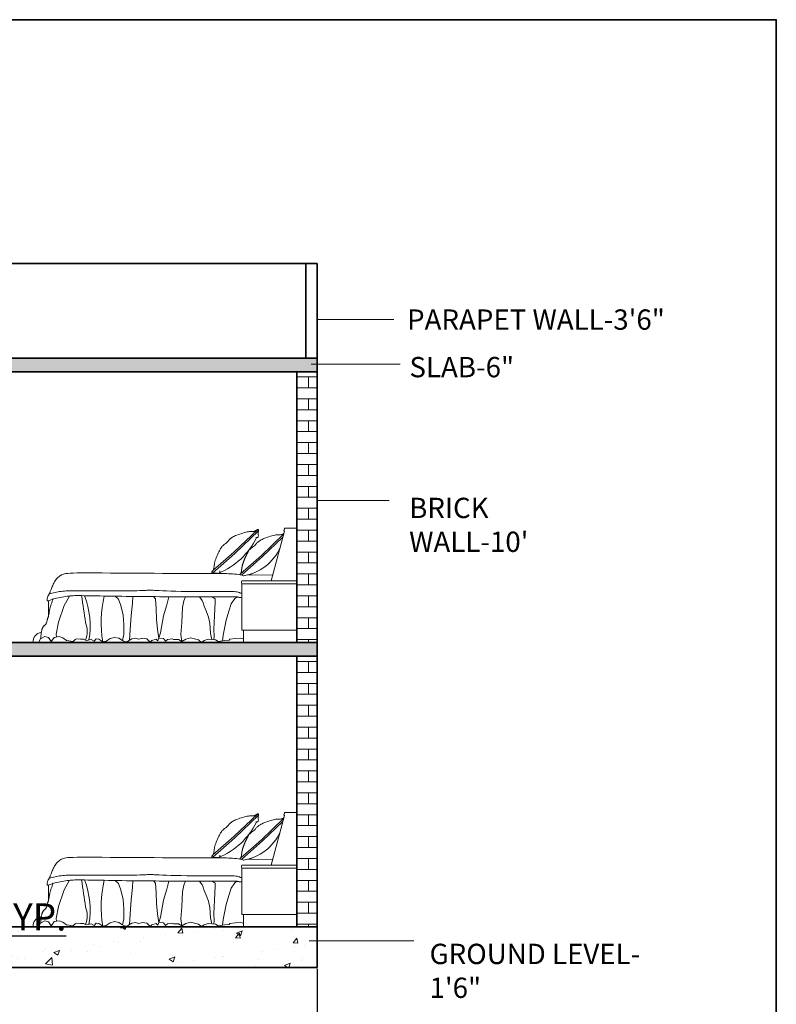
# Model space of a CAD drawing. Units: inches. Extents: x 2142 to 3604, y 1690 to 2981.
# Tile 9 of 9: x 3269 to 3604, y 2545 to 2981. Entities that reach past the tile are written whole.
import ezdxf

# ---------------------------------------------------------------- set-up
doc = ezdxf.new("R2010")
doc.units = ezdxf.units.IN
for name, color, linetype, lineweight in [('A-ANNO-DIMS', 2, 'Continuous', 18), ('A-ANNO-TEXT', 7, 'Continuous', 18), ('A-ANNO-TTLB', 7, 'Continuous', 35), ('A-FLOR-PATT', 8, 'Continuous', 13), ('A-FURN', 8, 'Continuous', 18), ('A-SECT', 7, 'Continuous', 35), ('A-WALL-PATT', 8, 'Continuous', 13)]:
    doc.layers.add(name, color=color, linetype=linetype, lineweight=lineweight)
doc.styles.get("Standard").update_dxf_attribs({"font": 'arial.ttf'})
doc.dimstyles.new('ISO-25', dxfattribs={"dimtxt": 12, "dimasz": 2.5, "dimexe": 1.25, "dimexo": 0.625, "dimtad": 1, "dimdec": 0, "dimlunit": 3, "dimtxsty": 'Standard', "dimcen": 2.5, "dimadec": 0, "dimazin": 0, "dimtfac": 1, "dimtdec": 0, "dimtmove": 0, "dimatfit": 3, "dimfxl": 1, "dimarcsym": 0})

# ---------------------------------------------------------------- blocks, each defined once
blk = doc.blocks.new('A$C08BC4B9A')
for p, q in [((0, 924.5), (0.5, 925)), ((0, 0), (0, 924.5)), ((95, 925), (0.5, 925)), ((101.1, 921.9), (105, 907.4)), ((101.4, 901.2), (208.9, 500)), ((106.6, 881.7), (106.8, 881.6)), ((106.8, 881.6), (109.7, 879.8)), ((109.7, 879.8), (112.8, 878.1)), ((112.8, 878.1), (116.3, 876.5)), ((311.4, 909.3), (311.5, 910.8)), ((311.5, 907.6), (311.4, 909.3)), ((311.5, 910.8), (311.7, 912.1)), ((311.7, 905.6), (311.5, 907.6)), ((311.7, 912.1), (312.1, 913.2)), ((312, 903.5), (311.7, 905.6)), ((502.9, 721.7), (311.9, 904.5)), ((312.3, 901.1), (312, 903.5)), ((312.1, 913.2), (312.7, 914.1)), ((312.6, 898.6), (312.3, 901.1)), ((312.9, 895.9), (312.6, 898.6)), ((312.7, 914.1), (313.6, 914.7)), ((313.1, 892.9), (312.9, 895.9)), ((313.3, 889.8), (313.1, 892.9)), ((313.4, 886.5), (313.3, 889.8)), ((313.3, 875.5), (313.4, 879.4)), ((313.4, 883), (313.4, 886.5)), ((313.4, 879.4), (313.4, 883)), ((313.6, 914.7), (314.7, 915)), ((314.7, 915), (316, 915.1)), ((316, 915.1), (317.6, 914.9)), ((317.6, 914.9), (319.3, 914.5)), ((319.3, 914.5), (321.1, 913.7)), ((511.6, 731.1), (320.5, 913.9)), ((321.1, 913.7), (323.2, 912.6)), ((323.2, 912.6), (325.4, 911.2)), ((325.4, 911.2), (327.8, 909.6)), ((327.8, 909.6), (330.4, 907.8)), ((330.4, 907.8), (333.3, 906.1)), ((333.3, 906.1), (336.4, 904.3)), ((336.4, 904.3), (339.9, 902.7)), ((339.9, 902.7), (343.7, 901.4)), ((343.7, 901.4), (347.9, 900.4)), ((347.9, 900.4), (352.5, 899.8)), ((352.5, 899.8), (357.6, 899.5)), ((357.6, 899.5), (363.2, 899.4)), ((363.2, 899.4), (369.6, 899.2)), ((369.6, 899.2), (376.7, 898.9)), ((376.7, 898.9), (384.6, 898.3)), ((384.6, 898.3), (393.4, 897.3)), ((393.4, 897.3), (403.3, 895.7)), ((403.3, 895.7), (414.2, 893.3)), ((414.2, 893.3), (425.9, 890.4)), ((425.9, 890.4), (438.1, 886.9)), ((438.1, 886.9), (450.5, 883.1)), ((450.5, 883.1), (462.9, 878.9)), ((462.9, 878.9), (474.9, 874.6)), ((288, 704.9), (107.8, 877.3)), ((279.2, 695.5), (114.2, 853.4)), ((116.3, 876.5), (120.1, 875.2)), ((120.1, 875.2), (124.3, 874.2)), ((124.3, 874.2), (128.9, 873.6)), ((128.9, 873.6), (134, 873.3)), ((134, 873.3), (139.6, 873.2)), ((139.6, 873.2), (146, 873)), ((146, 873), (153.1, 872.7)), ((153.1, 872.7), (161, 872.1)), ((161, 872.1), (169.8, 871.1)), ((169.8, 871.1), (179.7, 869.5)), ((179.7, 869.5), (190.6, 867.1)), ((190.6, 867.1), (202.3, 864.2)), ((202.3, 864.2), (214.5, 860.7)), ((214.5, 860.7), (226.9, 856.8)), ((226.9, 856.8), (239.3, 852.7)), ((239.3, 852.7), (251.3, 848.4)), ((251.3, 848.4), (262.7, 844)), ((262.7, 844), (273.2, 839.6)), ((273.2, 839.6), (282.5, 835.5)), ((282.5, 835.5), (290.7, 831.4)), ((290.7, 831.4), (298, 827.4)), ((298, 827.4), (304.4, 823.4)), ((304.4, 823.4), (310.1, 819.5)), ((310.1, 819.5), (315.2, 815.4)), ((312.7, 863.2), (312.8, 867.3)), ((313.1, 859.2), (312.7, 863.2)), ((312.8, 867.3), (313, 871.5)), ((313, 871.5), (313.3, 875.5)), ((314.3, 855.7), (313.1, 859.2)), ((316.7, 852.8), (314.3, 855.7)), ((315.2, 815.4), (319.8, 811.3)), ((320.4, 850.8), (316.7, 852.8)), ((319.8, 811.3), (324.1, 807)), ((325.8, 849.7), (320.4, 850.8)), ((324.1, 807), (328.1, 802.5)), ((333.2, 849.9), (325.8, 849.7)), ((328.1, 802.5), (332, 797.9)), ((332, 797.9), (335.8, 793.2)), ((474.9, 874.6), (486.3, 870.2)), ((486.3, 870.2), (496.8, 865.9)), ((496.8, 865.9), (506.1, 861.7)), ((506.1, 861.7), (514.3, 857.6)), ((514.3, 857.6), (521.6, 853.6)), ((521.6, 853.6), (528, 849.7)), ((528, 849.7), (533.7, 845.7)), ((533.7, 845.7), (538.8, 841.7)), ((538.8, 841.7), (543.4, 837.5)), ((543.4, 837.5), (547.7, 833.2)), ((547.7, 833.2), (551.7, 828.7)), ((551.7, 828.7), (555.6, 824.1)), ((555.6, 824.1), (559.4, 819.4)), ((559.4, 819.4), (563.3, 814.6)), ((563.3, 814.6), (567.7, 810.4)), ((572.2, 806.3), (567.7, 810.4)), ((577.3, 802.8), (572.2, 806.3)), ((582.3, 799.4), (577.3, 802.8)), ((587.2, 795.8), (582.3, 799.4)), ((335.8, 793.2), (339.7, 788.4)), ((339.7, 788.4), (344.1, 784.1)), ((344.2, 784), (344.1, 784.1)), ((344.5, 783.8), (344.2, 784)), ((344.9, 783.4), (344.5, 783.8)), ((345.5, 782.9), (344.9, 783.4)), ((346.1, 782.3), (345.5, 782.9)), ((346.8, 781.7), (346.1, 782.3)), ((347.6, 781.1), (346.8, 781.7)), ((348.3, 780.5), (347.6, 781.1)), ((349.1, 779.9), (348.3, 780.5)), ((349.8, 779.4), (349.1, 779.9)), ((350.5, 778.9), (349.8, 779.4)), ((351.1, 778.4), (350.5, 778.9)), ((351.8, 777.9), (351.1, 778.4)), ((352.4, 777.5), (351.8, 777.9)), ((353.1, 777), (352.4, 777.5)), ((353.7, 776.6), (353.1, 777)), ((354.3, 776.2), (353.7, 776.6)), ((354.9, 775.7), (354.3, 776.2)), ((355.6, 775.3), (354.9, 775.7)), ((356.2, 774.9), (355.6, 775.3)), ((356.8, 774.4), (356.2, 774.9)), ((357.4, 774), (356.8, 774.4)), ((358.1, 773.6), (357.4, 774)), ((358.7, 773.1), (358.1, 773.6)), ((359.3, 772.7), (358.7, 773.1)), ((359.9, 772.3), (359.3, 772.7)), ((360.5, 771.8), (359.9, 772.3)), ((361.2, 771.4), (360.5, 771.8)), ((361.8, 770.9), (361.2, 771.4)), ((362.4, 770.5), (361.8, 770.9)), ((363, 770), (362.4, 770.5)), ((363.6, 769.6), (363, 770)), ((364.2, 769.1), (363.6, 769.6)), ((364.8, 768.7), (364.2, 769.1)), ((365.4, 768.2), (364.8, 768.7)), ((366, 767.8), (365.4, 768.2)), ((366.6, 767.3), (366, 767.8)), ((367.2, 766.8), (366.6, 767.3)), ((367.8, 766.4), (367.2, 766.8)), ((368.3, 765.9), (367.8, 766.4)), ((368.9, 765.4), (368.3, 765.9)), ((369.5, 764.9), (368.9, 765.4)), ((370.1, 764.4), (369.5, 764.9)), ((370.7, 763.9), (370.1, 764.4)), ((371.2, 763.5), (370.7, 763.9)), ((371.8, 763), (371.2, 763.5)), ((372.4, 762.4), (371.8, 763)), ((373, 761.9), (372.4, 762.4)), ((373.5, 761.4), (373, 761.9)), ((374.1, 760.9), (373.5, 761.4)), ((374.7, 760.4), (374.1, 760.9)), ((375.2, 759.8), (374.7, 760.4)), ((375.8, 759.3), (375.2, 759.8)), ((376.3, 758.7), (375.8, 759.3)), ((376.9, 758.2), (376.3, 758.7)), ((377.4, 757.6), (376.9, 758.2)), ((378, 757), (377.4, 757.6)), ((378.6, 756.5), (378, 757)), ((379.2, 755.8), (378.6, 756.5)), ((379.8, 755.2), (379.2, 755.8)), ((380.5, 754.5), (379.8, 755.2)), ((381.3, 753.8), (380.5, 754.5)), ((382.2, 753.1), (381.3, 753.8)), ((383.2, 752.3), (382.2, 753.1)), ((384.2, 751.4), (383.2, 752.3)), ((385.4, 750.5), (384.2, 751.4)), ((386.6, 749.6), (385.4, 750.5)), ((387.8, 748.7), (386.6, 749.6)), ((388.9, 747.8), (387.8, 748.7)), ((389.9, 746.9), (388.9, 747.8)), ((390.8, 746), (389.9, 746.9)), ((391.4, 745.3), (390.8, 746)), ((391.9, 744.6), (391.4, 745.3)), ((392.1, 744), (391.9, 744.6)), ((392, 741.9), (392.1, 742.4)), ((392, 741.3), (392, 741.9)), ((392, 740.8), (392, 741.3)), ((392.1, 740.1), (392, 740.8)), ((392.2, 743.4), (392.1, 744)), ((392.1, 742.4), (392.2, 742.9)), ((392.4, 739.4), (392.1, 740.1)), ((392.2, 742.9), (392.2, 743.4)), ((392.7, 738.6), (392.4, 739.4)), ((393.1, 737.8), (392.7, 738.6)), ((393.6, 737), (393.1, 737.8)), ((394.1, 736.1), (393.6, 737)), ((394.7, 735.2), (394.1, 736.1)), ((395.2, 734.3), (394.7, 735.2)), ((395.8, 733.4), (395.2, 734.3)), ((396.4, 732.4), (395.8, 733.4)), ((397, 731.5), (396.4, 732.4)), ((397.6, 730.5), (397, 731.5)), ((398.2, 729.5), (397.6, 730.5)), ((398.7, 728.5), (398.2, 729.5)), ((399.3, 727.4), (398.7, 728.5)), ((399.9, 726.4), (399.3, 727.4)), ((400.5, 725.3), (399.9, 726.4)), ((401.1, 724.3), (400.5, 725.3)), ((401.7, 723.2), (401.1, 724.3)), ((402.4, 722), (401.7, 723.2)), ((403, 720.9), (402.4, 722)), ((403.6, 719.8), (403, 720.9)), ((404.2, 718.6), (403.6, 719.8)), ((404.8, 717.4), (404.2, 718.6)), ((685.7, 562.3), (502.9, 721.7)), ((681.3, 583.2), (511.6, 731.1)), ((592, 792.2), (587.2, 795.8)), ((596.6, 788.2), (592, 792.2)), ((601.1, 783.9), (596.6, 788.2)), ((605.5, 779.1), (601.1, 783.9)), ((609.9, 773.7), (605.5, 779.1)), ((614.3, 767.6), (609.9, 773.7)), ((618.8, 760.7), (614.3, 767.6)), ((623.5, 752.8), (618.8, 760.7)), ((628.4, 743.8), (623.5, 752.8)), ((633.5, 733.7), (628.4, 743.8)), ((638.7, 722.7), (633.5, 733.7)), ((643.9, 711), (638.7, 722.7)), ((450.1, 546.6), (279.2, 695.5)), ((457.7, 557), (288, 704.9)), ((405.4, 716.2), (404.8, 717.4)), ((406.1, 715), (405.4, 716.2)), ((406.7, 713.8), (406.1, 715)), ((407.3, 712.5), (406.7, 713.8)), ((408, 711.2), (407.3, 712.5)), ((408.6, 710), (408, 711.2)), ((409.3, 708.7), (408.6, 710)), ((409.9, 707.3), (409.3, 708.7)), ((410.6, 706), (409.9, 707.3)), ((411.2, 704.7), (410.6, 706)), ((411.9, 703.3), (411.2, 704.7)), ((412.5, 701.9), (411.9, 703.3)), ((413.2, 700.6), (412.5, 701.9)), ((413.8, 699.2), (413.2, 700.6)), ((414.5, 697.8), (413.8, 699.2)), ((415.1, 696.4), (414.5, 697.8)), ((415.8, 694.9), (415.1, 696.4)), ((416.4, 693.5), (415.8, 694.9)), ((417.1, 692.1), (416.4, 693.5)), ((417.7, 690.6), (417.1, 692.1)), ((418.4, 689.2), (417.7, 690.6)), ((419, 687.7), (418.4, 689.2)), ((419.7, 686.2), (419, 687.7)), ((420.3, 684.7), (419.7, 686.2)), ((421, 683.3), (420.3, 684.7)), ((421.6, 681.8), (421, 683.3)), ((422.2, 680.3), (421.6, 681.8)), ((422.9, 678.8), (422.2, 680.3)), ((423.5, 677.3), (422.9, 678.8)), ((424.1, 675.8), (423.5, 677.3)), ((424.7, 674.3), (424.1, 675.8)), ((425.4, 672.8), (424.7, 674.3)), ((426, 671.3), (425.4, 672.8)), ((426.6, 669.7), (426, 671.3)), ((427.2, 668.2), (426.6, 669.7)), ((427.8, 666.7), (427.2, 668.2)), ((428.4, 665.2), (427.8, 666.7)), ((429, 663.7), (428.4, 665.2)), ((429.6, 662.2), (429, 663.7)), ((430.1, 660.7), (429.6, 662.2)), ((430.7, 659.2), (430.1, 660.7)), ((431.3, 657.7), (430.7, 659.2)), ((431.8, 656.2), (431.3, 657.7)), ((432.4, 654.7), (431.8, 656.2)), ((432.9, 653.2), (432.4, 654.7)), ((433.4, 651.8), (432.9, 653.2)), ((434, 650.3), (433.4, 651.8)), ((434.5, 648.8), (434, 650.3)), ((435, 647.4), (434.5, 648.8)), ((435.5, 645.9), (435, 647.4)), ((436, 644.5), (435.5, 645.9)), ((436.5, 643.1), (436, 644.5)), ((436.9, 641.7), (436.5, 643.1)), ((437.4, 640.2), (436.9, 641.7)), ((437.9, 638.8), (437.4, 640.2)), ((438.3, 637.5), (437.9, 638.8)), ((649, 699), (643.9, 711)), ((653.8, 686.9), (649, 699)), ((658.2, 675), (653.8, 686.9)), ((662, 663.6), (658.2, 675)), ((665.2, 652.9), (662, 663.6)), ((667.5, 643.2), (665.2, 652.9)), ((669.2, 634.4), (667.5, 643.2)), ((438.7, 636.1), (438.3, 637.5)), ((439.1, 634.7), (438.7, 636.1)), ((439.6, 633.4), (439.1, 634.7)), ((440, 632), (439.6, 633.4)), ((440.3, 630.7), (440, 632)), ((440.7, 629.4), (440.3, 630.7)), ((441.1, 628.1), (440.7, 629.4)), ((441.4, 626.8), (441.1, 628.1)), ((441.8, 625.5), (441.4, 626.8)), ((442.1, 624.3), (441.8, 625.5)), ((442.4, 623.1), (442.1, 624.3)), ((442.7, 621.8), (442.4, 623.1)), ((443, 620.6), (442.7, 621.8)), ((443.3, 619.4), (443, 620.6)), ((443.6, 618.3), (443.3, 619.4)), ((443.8, 617.1), (443.6, 618.3)), ((444.1, 616), (443.8, 617.1)), ((444.3, 614.8), (444.1, 616)), ((444.5, 613.7), (444.3, 614.8)), ((444.7, 612.6), (444.5, 613.7)), ((445, 611.5), (444.7, 612.6)), ((445.2, 610.5), (445, 611.5)), ((445.4, 609.4), (445.2, 610.5)), ((445.5, 608.4), (445.4, 609.4)), ((445.7, 607.3), (445.5, 608.4)), ((445.9, 606.3), (445.7, 607.3)), ((446, 605.3), (445.9, 606.3)), ((446.2, 604.3), (446, 605.3)), ((446.4, 603.3), (446.2, 604.3)), ((446.5, 602.4), (446.4, 603.3)), ((446.6, 601.4), (446.5, 602.4)), ((446.8, 600.5), (446.6, 601.4)), ((446.9, 599.6), (446.8, 600.5)), ((447, 598.6), (446.9, 599.6)), ((447.1, 597.7), (447, 598.6)), ((447.2, 596.9), (447.1, 597.7)), ((447.3, 596), (447.2, 596.9)), ((447.4, 595.1), (447.3, 596)), ((447.5, 594.3), (447.4, 595.1)), ((447.6, 593.4), (447.5, 594.3)), ((447.7, 592.6), (447.6, 593.4)), ((447.8, 591.8), (447.7, 592.6)), ((447.9, 591), (447.8, 591.8)), ((448, 590.2), (447.9, 591)), ((448, 589.4), (448, 590.2)), ((448.1, 588.6), (448, 589.4)), ((448.2, 587.9), (448.1, 588.6)), ((448.3, 587.1), (448.2, 587.9)), ((448.3, 586.4), (448.3, 587.1)), ((448.4, 585.6), (448.3, 586.4)), ((448.5, 584.9), (448.4, 585.6)), ((448.6, 584.2), (448.5, 584.9)), ((448.6, 583.5), (448.6, 584.2)), ((448.7, 582.8), (448.6, 583.5)), ((448.8, 582.1), (448.7, 582.8)), ((448.9, 581.4), (448.8, 582.1)), ((448.9, 580.8), (448.9, 581.4)), ((449, 580.1), (448.9, 580.8)), ((449.1, 579.5), (449, 580.1)), ((449.2, 578.8), (449.1, 579.5)), ((449.3, 578.2), (449.2, 578.8)), ((449.4, 577.6), (449.3, 578.2)), ((449.5, 577), (449.4, 577.6)), ((449.6, 576.4), (449.5, 577)), ((449.7, 575.8), (449.6, 576.4)), ((449.8, 575.2), (449.7, 575.8)), ((449.9, 574.6), (449.8, 575.2)), ((450, 574), (449.9, 574.6)), ((450.1, 573.5), (450, 574)), ((450.3, 572.9), (450.1, 573.5)), ((450.4, 572.4), (450.3, 572.9)), ((450.5, 571.8), (450.4, 572.4)), ((450.7, 571.3), (450.5, 571.8)), ((450.8, 570.8), (450.7, 571.3)), ((451, 570.2), (450.8, 570.8)), ((451.1, 569.7), (451, 570.2)), ((451.3, 569.2), (451.1, 569.7)), ((451.5, 568.7), (451.3, 569.2)), ((451.6, 568.2), (451.5, 568.7)), ((451.8, 567.7), (451.6, 568.2)), ((452, 567.2), (451.8, 567.7)), ((452.2, 566.8), (452, 567.2)), ((452.4, 566.3), (452.2, 566.8)), ((452.6, 565.8), (452.4, 566.3)), ((452.8, 565.4), (452.6, 565.8)), ((453, 564.9), (452.8, 565.4)), ((453.2, 564.5), (453, 564.9)), ((453.4, 564), (453.2, 564.5)), ((453.6, 563.6), (453.4, 564)), ((453.8, 563.1), (453.6, 563.6)), ((454.1, 562.7), (453.8, 563.1)), ((454.3, 562.3), (454.1, 562.7)), ((454.5, 561.9), (454.3, 562.3)), ((454.8, 561.5), (454.5, 561.9)), ((455, 561.1), (454.8, 561.5)), ((455.2, 560.7), (455, 561.1)), ((455.5, 560.3), (455.2, 560.7)), ((455.7, 559.9), (455.5, 560.3)), ((456, 559.5), (455.7, 559.9)), ((456.2, 559.1), (456, 559.5)), ((456.4, 558.8), (456.2, 559.1)), ((456.7, 558.4), (456.4, 558.8)), ((586, 558.6), (569.7, 558.1)), ((603.2, 559), (586, 558.6)), ((621.8, 559.3), (603.2, 559)), ((642.6, 559.5), (621.8, 559.3)), ((624.8, 579.5), (625.2, 572.1)), ((625.2, 572.1), (626.6, 566.8)), ((626.6, 566.8), (629, 563.3)), ((629, 563.3), (632, 561.2)), ((632, 561.2), (635.6, 560.2)), ((635.6, 560.2), (639.6, 560.1)), ((639.6, 560.1), (643.7, 560.5)), ((666.5, 559.6), (642.6, 559.5)), ((643.7, 560.5), (647.9, 561)), ((647.9, 561), (651.9, 561.6)), ((651.9, 561.6), (655.7, 562)), ((655.7, 562), (659.3, 562.3)), ((659.3, 562.3), (662.8, 562.5)), ((662.8, 562.5), (666.1, 562.7)), ((666.1, 562.7), (669.2, 562.7)), ((693.9, 559.6), (666.5, 559.6)), ((670.4, 626.6), (669.2, 634.4)), ((669.2, 562.7), (672.2, 562.7)), ((671.3, 619.5), (670.4, 626.6)), ((671.9, 613.2), (671.3, 619.5)), ((672.5, 607.6), (671.9, 613.2)), ((672.2, 562.7), (674.9, 562.7)), ((673.1, 602.5), (672.5, 607.6)), ((674.1, 598), (673.1, 602.5)), ((675.4, 593.9), (674.1, 598)), ((674.9, 562.7), (677.5, 562.6)), ((677, 590.2), (675.4, 593.9)), ((678.8, 586.8), (677, 590.2)), ((677.5, 562.6), (679.8, 562.4)), ((680.8, 583.8), (678.8, 586.8)), ((679.8, 562.4), (682, 562.3)), ((682.8, 581.1), (680.8, 583.8)), ((682, 562.3), (683.9, 562.3)), ((684.7, 578.6), (682.8, 581.1)), ((683.9, 562.3), (685.7, 562.3)), ((686.5, 576.4), (684.7, 578.6)), ((685.7, 562.3), (687.2, 562.4)), ((688.1, 574.3), (686.5, 576.4)), ((687.2, 562.4), (688.5, 562.7)), ((689.3, 572.3), (688.1, 574.3)), ((688.5, 562.7), (689.5, 563.2)), ((690.2, 570.5), (689.3, 572.3)), ((689.5, 563.2), (690.3, 563.9)), ((690.8, 568.8), (690.2, 570.5)), ((690.3, 563.9), (690.9, 564.9)), ((691.1, 567.3), (690.8, 568.8)), ((690.9, 564.9), (691.1, 566)), ((691.1, 566), (691.1, 567.3)), ((725.8, 559.7), (693.9, 559.6)), ((762.8, 559.7), (725.8, 559.7)), ((805.4, 559.7), (762.8, 559.7)), ((853.4, 559.7), (805.4, 559.7)), ((906.2, 559.7), (853.4, 559.7)), ((963.4, 559.8), (906.2, 559.7)), ((1024.6, 559.9), (963.4, 559.8)), ((1089.2, 560.1), (1024.6, 559.9)), ((1156.7, 560.4), (1089.2, 560.1)), ((1226.8, 560.7), (1156.7, 560.4)), ((1298.7, 561.1), (1226.8, 560.7)), ((1371.2, 561.6), (1298.7, 561.1)), ((1443.1, 562.1), (1371.2, 561.6)), ((1512.8, 562.6), (1443.1, 562.1)), ((1579.1, 563), (1512.8, 562.6)), ((1640.5, 563.3), (1579.1, 563)), ((1695.8, 563.4), (1640.5, 563.3)), ((1743.5, 563.3), (1695.8, 563.4)), ((1782.8, 563), (1743.5, 563.3)), ((1814.2, 562.4), (1782.8, 563)), ((1838.9, 561.5), (1814.2, 562.4)), ((1858, 560.2), (1838.9, 561.5)), ((1872.6, 558.6), (1858, 560.2)), ((1883.7, 556.6), (1872.6, 558.6)), ((445.9, 500), (0, 500)), ((366.1, 546.8), (196.6, 546.1)), ((400.7, 547.5), (366.1, 546.8)), ((420, 543.6), (400.7, 547.5)), ((431.7, 540.1), (420, 543.6)), ((439.4, 542.5), (431.7, 540.1)), ((445.4, 545.7), (439.4, 542.5)), ((460.2, 548.4), (445.4, 545.7)), ((456.9, 558), (456.7, 558.4)), ((457.2, 557.7), (456.9, 558)), ((457.4, 557.3), (457.2, 557.7)), ((457.7, 557), (457.4, 557.3)), ((457.9, 556.6), (457.7, 557)), ((458.2, 556.3), (457.9, 556.6)), ((458.4, 555.9), (458.2, 556.3)), ((458.7, 555.6), (458.4, 555.9)), ((458.9, 555.3), (458.7, 555.6)), ((459.2, 554.9), (458.9, 555.3)), ((459.4, 554.6), (459.2, 554.9)), ((459.7, 554.3), (459.4, 554.6)), ((459.9, 554), (459.7, 554.3)), ((460.2, 553.6), (459.9, 554)), ((460.4, 553.3), (460.2, 553.6)), ((475.2, 550.7), (460.2, 548.4)), ((460.7, 553), (460.4, 553.3)), ((461, 552.6), (460.7, 553)), ((461.3, 552.3), (461, 552.6)), ((461.6, 551.9), (461.3, 552.3)), ((461.9, 551.5), (461.6, 551.9)), ((462.2, 551.1), (461.9, 551.5)), ((462.5, 550.7), (462.2, 551.1)), ((462.8, 550.3), (462.5, 550.7)), ((463.2, 549.8), (462.8, 550.3)), ((463.5, 549.4), (463.2, 549.8)), ((463.8, 548.9), (463.5, 549.4)), ((490.5, 552.6), (475.2, 550.7)), ((506, 554.2), (490.5, 552.6)), ((521.7, 555.5), (506, 554.2)), ((537.6, 556.6), (521.7, 555.5)), ((553.6, 557.4), (537.6, 556.6)), ((569.7, 558.1), (553.6, 557.4)), ((1892.6, 554.2), (1883.7, 556.6)), ((1900.3, 551.3), (1892.6, 554.2)), ((1907.7, 547.9), (1900.3, 551.3)), ((1915, 544), (1907.7, 547.9)), ((1922.1, 539.6), (1915, 544)), ((1929, 534.5), (1922.1, 539.6)), ((1935.8, 528.9), (1929, 534.5)), ((1942.3, 522.6), (1935.8, 528.9)), ((1948.6, 515.6), (1942.3, 522.6)), ((1954.6, 508), (1948.6, 515.6)), ((1960.4, 499.6), (1954.6, 508)), ((1965.8, 490.7), (1960.4, 499.6)), ((1970.9, 481.5), (1965.8, 490.7)), ((1975.6, 472.1), (1970.9, 481.5)), ((445.9, 475), (0, 475)), ((445.9, 475), (445.9, 100)), ((449.1, 398.3), (453.4, 399.2)), ((453.4, 399.2), (457.6, 400.4)), ((457.6, 400.4), (461.8, 402)), ((461.8, 402), (466.2, 403.7)), ((466.2, 403.7), (471.3, 405.6)), ((471.3, 405.6), (477.6, 407.5)), ((477.6, 407.5), (485.4, 409.4)), ((485.4, 409.4), (495.3, 411.1)), ((495.3, 411.1), (507.7, 412.5)), ((507.7, 412.5), (523, 413.5)), ((523, 413.5), (541.5, 414)), ((541.5, 414), (563.2, 414.2)), ((563.2, 414.2), (588.2, 414.1)), ((588.2, 414.1), (616.4, 413.7)), ((616.4, 413.7), (647.7, 413.3)), ((647.7, 413.3), (682, 412.9)), ((682, 412.9), (719.4, 412.6)), ((719.4, 412.6), (759.7, 412.4)), ((759.7, 412.4), (802.6, 412.6)), ((802.6, 412.6), (847.4, 413)), ((847.4, 413), (892.8, 413.6)), ((892.8, 413.6), (937.8, 414.4)), ((937.8, 414.4), (981.1, 415.3)), ((981.1, 415.3), (1021.7, 416.4)), ((1021.7, 416.4), (1058.6, 417.5)), ((1058.6, 417.5), (1090.4, 418.7)), ((1090.4, 418.7), (1116.5, 419.9)), ((1116.5, 419.9), (1137.2, 421)), ((1137.2, 421), (1153.4, 422.1)), ((1153.4, 422.1), (1165.7, 423)), ((1165.7, 423), (1174.9, 423.8)), ((1174.9, 423.8), (1181.7, 424.4)), ((1181.7, 424.4), (1186.9, 424.8)), ((1186.9, 424.8), (1191.2, 425)), ((1191.2, 425), (1195.4, 424.8)), ((1195.4, 424.8), (1200, 424.5)), ((1200, 424.5), (1205.8, 423.9)), ((1205.8, 423.9), (1213.3, 423.2)), ((1213.3, 423.2), (1223.1, 422.4)), ((1223.1, 422.4), (1236, 421.7)), ((1236, 421.7), (1252.5, 420.9)), ((1252.5, 420.9), (1273.3, 420.3)), ((1273.3, 420.3), (1298.7, 419.7)), ((1298.7, 419.7), (1328.3, 419.4)), ((1328.3, 419.4), (1361.1, 419.1)), ((1361.1, 419.1), (1396.4, 418.9)), ((1396.4, 418.9), (1433.4, 418.8)), ((1433.4, 418.8), (1471.3, 418.7)), ((1471.3, 418.7), (1509.3, 418.7)), ((1509.3, 418.7), (1546.6, 418.7)), ((1546.6, 418.7), (1582.4, 418.7)), ((1582.4, 418.7), (1616.7, 418.7)), ((1616.7, 418.7), (1649.3, 418.7)), ((1649.3, 418.7), (1680.1, 418.7)), ((1680.1, 418.7), (1709, 418.7)), ((1709, 418.7), (1736, 418.7)), ((1736, 418.7), (1760.9, 418.7)), ((1760.9, 418.7), (1783.8, 418.7)), ((1783.8, 418.7), (1804.5, 418.7)), ((1804.5, 418.7), (1823.2, 418.6)), ((1823.2, 418.6), (1840.3, 418.5)), ((1840.3, 418.5), (1856.1, 418.1)), ((1856.1, 418.1), (1870.7, 417.6)), ((1870.7, 417.6), (1884.5, 416.7)), ((1884.5, 416.7), (1897.8, 415.6)), ((1897.8, 415.6), (1910.8, 414)), ((1910.8, 414), (1923.7, 412)), ((1923.7, 412), (1936.5, 409.7)), ((1936.5, 409.7), (1949.1, 407.1)), ((1949.1, 407.1), (1961.3, 404.4)), ((1961.3, 404.4), (1973.1, 401.6)), ((1973.1, 401.6), (1984.4, 398.8)), ((1980, 462.7), (1975.6, 472.1)), ((1984, 453.6), (1980, 462.7)), ((1987.5, 445), (1984, 453.6)), ((1990.7, 437), (1987.5, 445)), ((1993.4, 429.7), (1990.7, 437)), ((1995.8, 423.3), (1993.4, 429.7)), ((1997.8, 417.5), (1995.8, 423.3)), ((1999.6, 412.4), (1997.8, 417.5)), ((2001.3, 407.8), (1999.6, 412.4)), ((2002.8, 403.7), (2001.3, 407.8)), ((2004.3, 400.1), (2002.8, 403.7)), ((2005.8, 396.8), (2004.3, 400.1)), ((445.9, 397.8), (449.1, 398.3)), ((445.9, 362), (481.5, 369.7)), ((445.9, 362.5), (450.4, 363.2)), ((450.4, 363.2), (457.2, 364.1)), ((457.2, 364.1), (463.4, 364.9)), ((463.4, 364.9), (468.9, 365.7)), ((468.9, 365.7), (473.6, 366.4)), ((473.6, 366.4), (477.6, 367.1)), ((477.6, 367.1), (481.1, 367.7)), ((481.1, 367.7), (484.4, 368.3)), ((484.4, 368.3), (488, 368.8)), ((504.7, 356.4), (486.2, 368.5)), ((488, 368.8), (492.3, 369.2)), ((492.3, 369.2), (497.5, 369.6)), ((497.5, 369.6), (504.1, 369.9)), ((504.1, 369.9), (512.5, 370.1)), ((534.3, 312.8), (504.7, 356.4)), ((512.5, 370.1), (522.9, 370.3)), ((522.9, 370.3), (535.3, 370.3)), ((535.3, 370.3), (549.5, 370.3)), ((549.5, 370.3), (565.4, 370.3)), ((565.4, 370.3), (582.8, 370.2)), ((582.8, 370.2), (601.6, 370.2)), ((601.6, 370.2), (621.6, 370.1)), ((621.6, 370.1), (642.7, 370.1)), ((642.7, 370.1), (664.7, 370.1)), ((663.6, 354.7), (661.8, 330.2)), ((661.8, 330.2), (668.8, 215.1)), ((687.3, 370.2), (663.6, 354.7)), ((664.7, 370.1), (687.3, 370.2)), ((687.3, 370.2), (710.4, 370.3)), ((710.4, 370.3), (733.4, 370.4)), ((733.4, 370.4), (756.3, 370.4)), ((750.9, 293.6), (759.6, 321.5)), ((756.3, 370.4), (778.7, 370.5)), ((759.6, 321.5), (768.3, 339)), ((768.3, 339), (789.4, 370.5)), ((778.7, 370.5), (800.2, 370.6)), ((800.2, 370.6), (820.7, 370.6)), ((820.7, 370.6), (840, 370.6)), ((840, 370.6), (858.3, 370.5)), ((858.3, 370.5), (876.2, 370.4)), ((876.2, 370.4), (894, 370.4)), ((894, 370.4), (912.3, 370.3)), ((916.7, 337.2), (903.2, 370.3)), ((912.3, 370.3), (931.5, 370.2)), ((927.2, 283.1), (916.7, 337.2)), ((931.5, 370.2), (952, 370.2)), ((952, 370.2), (974.3, 370.2)), ((974.3, 370.2), (998.7, 370.3)), ((998.7, 370.3), (1025.1, 370.4)), ((1025.1, 370.4), (1053.2, 370.6)), ((1054.7, 305.8), (1039.1, 370.5)), ((1053.2, 370.6), (1082.9, 370.8)), ((1082.9, 370.8), (1113.8, 371)), ((1113.8, 371), (1145.8, 371.3)), ((1145.5, 354.7), (1140.2, 274.4)), ((1162.2, 371.4), (1145.5, 354.7)), ((1145.8, 371.3), (1178.6, 371.6)), ((1178.6, 371.6), (1212, 371.9)), ((1212, 371.9), (1245.7, 372.2)), ((1245.7, 372.2), (1279.8, 372.6)), ((1279.8, 372.6), (1314.1, 373)), ((1314.1, 373), (1348.8, 373.4)), ((1332.3, 318), (1331.5, 373.2)), ((1348.8, 373.4), (1383.8, 373.8)), ((1383.8, 373.8), (1419.1, 374.3)), ((1419.1, 374.3), (1454.7, 374.8)), ((1428.3, 300.6), (1445.8, 351.2)), ((1445.8, 351.2), (1472.7, 375.1)), ((1454.7, 374.8), (1490.6, 375.4)), ((1490.6, 375.4), (1526.8, 376)), ((1526.8, 376), (1562.7, 376.6)), ((1562.7, 376.6), (1597.9, 377.2)), ((1597.9, 377.2), (1632, 377.8)), ((1632, 377.8), (1664.4, 378.4)), ((1664.4, 378.4), (1694.6, 378.9)), ((1694.6, 378.9), (1722.2, 379.3)), ((1722.2, 379.3), (1746.7, 379.5)), ((1746.7, 379.5), (1767.7, 379.7)), ((1767.7, 379.7), (1785.7, 379.6)), ((1785.7, 379.6), (1801.2, 379.4)), ((1801.2, 379.4), (1814.9, 378.9)), ((1814.9, 378.9), (1827.4, 378.2)), ((1827.4, 378.2), (1839.2, 377.2)), ((1839.2, 377.2), (1850.9, 375.9)), ((1845.1, 376.6), (1887, 298.9)), ((1850.9, 375.9), (1863.2, 374.3)), ((1863.2, 374.3), (1876.4, 372.4)), ((1876.4, 372.4), (1890.5, 370.2)), ((1890.5, 370.2), (1905, 367.7)), ((1905, 367.7), (1919.7, 364.9)), ((1919.7, 364.9), (1934.2, 362)), ((1934.2, 362), (1948.2, 358.9)), ((1948.2, 358.9), (1961.4, 355.7)), ((1961.4, 355.7), (1973.5, 352.4)), ((1973.5, 352.4), (1984.1, 349.1)), ((1977.1, 352.6), (1976.8, 353.5)), ((1978, 350), (1977.1, 352.6)), ((1979.4, 346.1), (1978, 350)), ((1981.2, 341.1), (1979.4, 346.1)), ((1983.2, 335.3), (1981.2, 341.1)), ((1985.5, 329), (1983.2, 335.3)), ((1984.1, 349.1), (1993.3, 345.9)), ((1984.4, 398.8), (1995, 396.1)), ((1987.8, 322.5), (1985.5, 329)), ((1990.1, 316.1), (1987.8, 322.5)), ((1993.3, 345.9), (2001.3, 342.9)), ((1995, 396.1), (2004.8, 393.6)), ((2001.3, 342.9), (2007.9, 340.5)), ((2007.5, 393.8), (2005.8, 396.8)), ((2009.2, 390.9), (2007.5, 393.8)), ((2007.9, 340.5), (2013.4, 338.6)), ((2010.9, 388.2), (2009.2, 390.9)), ((2012.7, 385.4), (2010.9, 388.2)), ((2014.5, 382.5), (2012.7, 385.4)), ((2013.4, 338.6), (2017.8, 337.5)), ((2016.4, 379.3), (2014.5, 382.5)), ((2015, 211.3), (2015, 338.2)), ((2018.2, 375.7), (2016.4, 379.3)), ((2017.8, 337.5), (2021.2, 337.3)), ((2020, 371.7), (2018.2, 375.7)), ((2021.7, 367.2), (2020, 371.7)), ((2021.2, 337.3), (2023.6, 338.3)), ((2023.2, 362.2), (2021.7, 367.2)), ((2024.6, 357.2), (2023.2, 362.2)), ((2023.6, 338.3), (2025.2, 340.5)), ((2025.5, 352.3), (2024.6, 357.2)), ((2025.2, 340.5), (2025.9, 343.7)), ((2026, 347.7), (2025.5, 352.3)), ((2025.9, 343.7), (2026, 347.7)), ((551.8, 253.5), (534.3, 312.8)), ((572.8, 180.2), (551.8, 253.5)), ((717.7, 206.4), (736.9, 257)), ((736.9, 257), (750.9, 293.6)), ((934.2, 161), (927.2, 283.1)), ((1082.6, 216.8), (1054.7, 305.8)), ((1140.2, 274.4), (1138.5, 188.9)), ((1342.8, 218.6), (1332.3, 318)), ((1409.1, 220.3), (1428.3, 300.6)), ((1887, 298.9), (1932.4, 164.5)), ((1992.3, 309.9), (1990.1, 316.1)), ((1994.4, 304), (1992.3, 309.9)), ((1996.4, 298.3), (1994.4, 304)), ((1998.2, 292.7), (1996.4, 298.3)), ((2000, 287.1), (1998.2, 292.7)), ((2001.6, 281.3), (2000, 287.1)), ((2003.1, 275.4), (2001.6, 281.3)), ((2004.5, 269.2), (2003.1, 275.4)), ((2005.8, 262.6), (2004.5, 269.2)), ((2006.9, 255.8), (2005.8, 262.6)), ((2008, 248.9), (2006.9, 255.8)), ((2009, 242.1), (2008, 248.9)), ((2010, 235.6), (2009, 242.1)), ((597.2, 59.8), (572.8, 180.2)), ((668.8, 215.1), (674, 106.9)), ((707.2, 155.8), (717.7, 206.4)), ((941.2, 65.1), (934.2, 161)), ((1105.3, 77.3), (1082.6, 216.8)), ((1138.5, 188.9), (1131.5, 105.2)), ((1353.2, 103.4), (1342.8, 218.6)), ((1403.9, 145.3), (1409.1, 220.3)), ((1932.4, 164.5), (1951.6, 66.8)), ((2011, 229.5), (2010, 235.6)), ((2011.9, 223.9), (2011, 229.5)), ((2012.9, 219), (2011.9, 223.9)), ((2013.9, 215), (2012.9, 219)), ((2014.9, 211.6), (2013.9, 215)), ((2015.9, 208.7), (2014.9, 211.6)), ((2017, 206), (2015.9, 208.7)), ((2018.1, 203.5), (2017, 206)), ((2019.2, 200.8), (2018.1, 203.5)), ((2020.3, 197.8), (2019.2, 200.8)), ((2021.4, 194.3), (2020.3, 197.8)), ((2022.5, 190.2), (2021.4, 194.3)), ((2023.7, 185.5), (2022.5, 190.2)), ((2024.9, 180.4), (2023.7, 185.5)), ((2026.1, 175.1), (2024.9, 180.4)), ((2027.4, 169.8), (2026.1, 175.1)), ((2028.9, 164.7), (2027.4, 169.8)), ((2030.5, 159.8), (2028.9, 164.7)), ((2032.2, 155.5), (2030.5, 159.8)), ((445.9, 100), (0, 100)), ((433.9, 100), (433.9, 0)), ((674, 106.9), (672.3, 47.6)), ((702, 72), (707.2, 155.8)), ((1131.5, 105.2), (1119, 34)), ((1356.3, 18.2), (1353.2, 103.4)), ((1403.9, 65.1), (1403.9, 145.3)), ((2034.1, 151.8), (2032.2, 155.5)), ((2036.1, 148.6), (2034.1, 151.8)), ((2038.3, 145.9), (2036.1, 148.6)), ((2040.5, 143.6), (2038.3, 145.9)), ((2042.8, 141.5), (2040.5, 143.6)), ((2045, 139.6), (2042.8, 141.5)), ((2047.3, 137.8), (2045, 139.6)), ((2049.5, 136), (2047.3, 137.8)), ((2051.6, 134.1), (2049.5, 136)), ((2053.6, 132), (2051.6, 134.1)), ((2055.6, 129.7), (2053.6, 132)), ((2057.4, 127.3), (2055.6, 129.7)), ((2059.1, 124.7), (2057.4, 127.3)), ((2060.8, 121.9), (2059.1, 124.7)), ((2062.3, 118.9), (2060.8, 121.9)), ((2063.8, 115.6), (2062.3, 118.9)), ((2065.1, 112), (2063.8, 115.6)), ((2066.4, 108.3), (2065.1, 112)), ((2067.5, 104.3), (2066.4, 108.3)), ((2068.6, 100.2), (2067.5, 104.3)), ((2069.5, 95.9), (2068.6, 100.2)), ((2070.4, 91.5), (2069.5, 95.9)), ((2071.2, 87), (2070.4, 91.5)), ((2072, 82.5), (2071.2, 87)), ((2072.6, 77.9), (2072, 82.5)), ((0, 0), (2150.5, 0)), ((433.9, 29.5), (455.7, 35.6)), ((455.7, 35.6), (497.9, 32.5)), ((497.9, 32.5), (543.3, 26.2)), ((543.3, 26.2), (549.6, 18.4)), ((549.6, 18.4), (587.1, 16.9)), ((587.1, 16.9), (618.4, 10.6)), ((602.8, 13.7), (597.2, 59.8)), ((618.4, 10.6), (638.7, 9)), ((638.7, 9), (660.6, 21.5)), ((660.6, 21.5), (720.1, 26.2)), ((672.3, 47.6), (674.3, 22.6)), ((690.4, 23.9), (702, 72)), ((720.1, 26.2), (752.9, 16.9)), ((752.9, 16.9), (773.3, 1.2)), ((773.3, 1.2), (798.3, 21.5)), ((798.3, 21.5), (864, 37.2)), ((864, 37.2), (900, 27.8)), ((900, 27.8), (932.8, 7.5)), ((932.8, 7.5), (941.2, 65.1)), ((932.8, 7.5), (961, 24.7)), ((961, 24.7), (1000.1, 23.1)), ((1000.1, 23.1), (1011.1, 29.4)), ((1011.1, 29.4), (1048.6, 23.1)), ((1048.6, 23.1), (1064.3, 10.6)), ((1064.3, 10.6), (1081.5, 32.5)), ((1081.5, 32.5), (1119, 34)), ((1119, 34), (1105.3, 77.3)), ((1119, 34), (1128.4, 12.2)), ((1128.4, 12.2), (1142.5, 26.2)), ((1142.5, 26.2), (1175.3, 16.9)), ((1175.3, 16.9), (1191, 2.8)), ((1191, 2.8), (1217.6, 29.4)), ((1217.6, 29.4), (1250.4, 35.6)), ((1250.4, 35.6), (1283.3, 26.2)), ((1283.3, 26.2), (1307.8, 35.4)), ((1307.8, 35.4), (1339.1, 29.2)), ((1339.1, 29.2), (1373.5, 7.3)), ((1373.5, 7.3), (1393.8, 5.7)), ((1393.8, 5.7), (1414.2, 16.7)), ((1414.2, 16.7), (1403.9, 65.1)), ((1414.2, 16.7), (1443.9, 33.9)), ((1443.9, 33.9), (1478.3, 41.7)), ((1478.3, 41.7), (1514.3, 32.3)), ((1514.3, 32.3), (1547.2, 10.4)), ((1547.2, 10.4), (1573.7, 5.7)), ((1573.7, 5.7), (1606.6, 26.1)), ((1606.6, 26.1), (1628.5, 29.2)), ((1628.5, 29.2), (1642.6, 10.4)), ((1642.6, 10.4), (1667.6, 24.5)), ((1667.6, 24.5), (1705.2, 16.7)), ((1705.2, 16.7), (1714.5, 18.2)), ((1714.5, 18.2), (1730.2, 27.6)), ((1730.2, 27.6), (1745.8, 27.6)), ((1745.8, 27.6), (1753.7, 27.6)), ((1753.7, 27.6), (1786.5, 30.7)), ((1786.5, 30.7), (1799, 24.5)), ((1799, 24.5), (1814.7, 8.9)), ((1814.7, 8.9), (1867.9, 15.1)), ((1867.9, 15.1), (1897.6, 37)), ((1897.6, 37), (1928.9, 47.9)), ((1928.9, 47.9), (1968, 41.7)), ((1951.6, 66.8), (1948.4, 44.8)), ((1968, 41.7), (1980.5, 21.4)), ((1980.5, 21.4), (1991.4, 8.9)), ((1991.4, 8.9), (2014.9, 40.1)), ((2014.9, 40.1), (2044.6, 47.9)), ((2044.6, 47.9), (2079, 30.7)), ((2073.3, 73.2), (2072.6, 77.9)), ((2073.9, 68.1), (2073.3, 73.2)), ((2074.7, 62.4), (2073.9, 68.1)), ((2075.5, 56), (2074.7, 62.4)), ((2076.5, 48.7), (2075.5, 56)), ((2077.6, 40.3), (2076.5, 48.7)), ((2079, 30.7), (2077.6, 40.3)), ((2079, 30.7), (2095.6, 0))]:
    blk.add_line(p, q)
for centre, radius, start, end in [((96.2, 920.6), 5, 15, 105), ((100.1, 906.1), 5, 285, 15), ((863.9, 1112.1), 597.2, 206.24729, 247.52644), ((487.1, 917.9), 380.4, 202.7795, 262.44771), ((429, 487.5), 21, 323.36963, 36.63037), ((634, 163.3), 952.9, 350.48063, 12.93386), ((2353.4, 135.1), 676.8, 158.84866, 189.74009), ((6455, -433.2), 4778, 170.20624, 172.85553), ((1887.2, 90.1), 187, 157.71552, 202.60163), ((2056.3, 0.1), 84.2, 359.90526, 78.73452)]:
    blk.add_arc(centre, radius, start, end)
blk = doc.blocks.new('*D76')
at = {"layer": 'A-ANNO-DIMS', "color": 0, "lineweight": -2, "transparency": 16777216}
for p, q in [((3164.16, 2578.5), (3164.16, 2573.76)), ((3166.66, 2575.01), (3183.23, 2575.01)), ((3185.73, 2578.5), (3185.73, 2573.76)), ((3185.73, 2575.01), (3289.46, 2575.01))]:
    blk.add_line(p, q, dxfattribs=at)
at = {"layer": 'A-ANNO-DIMS', "color": 0, "transparency": 16777216}
for points in [[(3166.66, 2575.43), (3166.66, 2574.59), (3164.16, 2575.01)], [(3183.23, 2575.43), (3183.23, 2574.59), (3185.73, 2575.01)]]:
    blk.add_solid(points, dxfattribs=at)
at = {"layer": 'Defpoints', "color": 0, "transparency": 16777216}
for p in [(3164.16, 2579.12), (3185.73, 2579.12), (3185.73, 2575.01)]:
    blk.add_point(p, dxfattribs=at)
at = {"layer": 'A-ANNO-DIMS', "color": 0, "transparency": 16777216, "insert": (3238.85, 2581.84), "char_height": 12, "attachment_point": 5}
blk.add_mtext('1\'-9 1/2" TYP.', dxfattribs=at)
blk = doc.blocks.new('*D93')
at = {"layer": 'A-ANNO-DIMS', "color": 0, "lineweight": -2, "transparency": 16777216}
for p, q in [((2923.33, 2560.39), (2923.33, 2526.72)), ((3400.83, 2560.39), (3400.83, 2526.72)), ((2925.83, 2527.97), (3398.33, 2527.97))]:
    blk.add_line(p, q, dxfattribs=at)
at = {"layer": 'A-ANNO-DIMS', "color": 0, "transparency": 16777216}
for points in [[(2925.83, 2528.38), (2925.83, 2527.55), (2923.33, 2527.97)], [(3398.33, 2528.38), (3398.33, 2527.55), (3400.83, 2527.97)]]:
    blk.add_solid(points, dxfattribs=at)
at = {"layer": 'Defpoints', "color": 0, "transparency": 16777216}
for p in [(2923.33, 2561.02), (3400.83, 2561.02), (3400.83, 2527.97)]:
    blk.add_point(p, dxfattribs=at)
at = {"layer": 'A-ANNO-DIMS', "color": 0, "transparency": 16777216, "insert": (3162.08, 2534.8), "char_height": 12, "attachment_point": 5}
blk.add_mtext('39\'-9 1/2"', dxfattribs=at)

msp = doc.modelspace()

# ---------------------------------------------------------------- hatches: boundary and pattern name
at = {"layer": 'A-FLOR-PATT'}
h = msp.add_hatch(dxfattribs=at)
h.set_pattern_fill('AR-CONC', color=256, scale=0.065, style=0)
h.paths.add_polyline_path([(2923.33, 2825.02), (3400.83, 2825.02), (3400.83, 2831.02), (2923.33, 2831.02)])
h = msp.add_hatch(dxfattribs=at)
h.set_pattern_fill('AR-CONC', color=256, scale=0.065, style=0)
h.paths.add_polyline_path([(2923.33, 2699.02), (3400.83, 2699.02), (3400.83, 2705.02), (2923.33, 2705.02)])
h = msp.add_hatch(dxfattribs=at)
h.set_pattern_fill('AR-CONC', color=256, scale=0.14, style=0)
h.paths.add_polyline_path([(2923.33, 2561.02), (3400.83, 2561.02), (3400.83, 2579.02), (2923.33, 2579.02)])
at = {"layer": 'A-WALL-PATT'}
h = msp.add_hatch(dxfattribs=at)
h.set_pattern_fill('AR-BRSTD', color=256, scale=0.0715954, style=0)
h.paths.add_polyline_path([(3391.83, 2705.02), (3400.83, 2705.02), (3400.83, 2825.02), (3391.83, 2825.02)])
h = msp.add_hatch(dxfattribs=at)
h.set_pattern_fill('AR-BRSTD', color=256, scale=0.0715954, style=0)
h.paths.add_polyline_path([(3391.83, 2579.02), (3400.83, 2579.02), (3400.83, 2699.02), (3391.83, 2699.02)])

# ---------------------------------------------------------------- linework, layer by layer
at = {"layer": 'A-ANNO-TEXT'}
for p, q in [((3400.83, 2848.1), (3434.87, 2848.1)), ((3398.18, 2828.32), (3437.68, 2828.32)), ((3400.83, 2767.87), (3432.8, 2767.87)), ((3397.29, 2572.82), (3443.61, 2572.82))]:
    msp.add_line(p, q, dxfattribs=at)
at = {"layer": 'A-ANNO-TTLB'}
msp.add_lwpolyline([(2142.1, 2981.01), (3604.42, 2981.01), (3604.42, 1690.13), (2142.1, 1690.13)], close=True, dxfattribs=at)
at = {"layer": 'A-SECT'}
for p, q in [((2923.33, 2873.02), (3400.83, 2873.02)), ((3395.73, 2831.02), (3395.73, 2873.02)), ((3400.83, 2873.02), (3400.83, 2687.02)), ((2923.33, 2831.02), (3400.83, 2831.02)), ((2923.33, 2825.02), (3400.83, 2825.02)), ((3391.83, 2825.02), (3391.83, 2705.02)), ((3400.83, 2747.02), (3400.83, 2561.02)), ((2923.33, 2705.02), (3400.83, 2705.02)), ((2923.33, 2699.02), (3400.83, 2699.02)), ((3391.83, 2699.02), (3391.83, 2579.02)), ((2923.33, 2579.02), (3400.83, 2579.02)), ((2923.33, 2561.02), (3400.83, 2561.02))]:
    msp.add_line(p, q, dxfattribs=at)

# ---------------------------------------------------------------- block references
at = {"layer": 'A-FURN', "xscale": -0.0546942147408242, "yscale": 0.0546942147408242, "zscale": 0.0546942147408242}
for p in [(3391.83, 2705.02), (3391.83, 2579.02)]:
    msp.add_blockref('A$C08BC4B9A', p, dxfattribs=at)

# ---------------------------------------------------------------- texts
at = {"layer": 'A-ANNO-TEXT', "char_height": 9, "attachment_point": 1}
for s, width, insert in [('PARAPET WALL-3\'6" ', 306.2115, (3440.68, 2852.62)), ('SLAB-6"', 70.605, (3441.73, 2831.55)), ("BRICK WALL-10'", 85.5819, (3441.6, 2769.15)), ('GROUND LEVEL- 1\'6"', 111.2882, (3450.65, 2571.51))]:
    msp.add_mtext_dynamic_manual_height_columns(s, width=width, gutter_width=12.5, heights=[0], dxfattribs=dict(at, insert=insert))

# ---------------------------------------------------------------- dimensions: what is measured, and where the dimension line sits
at = {"layer": 'A-ANNO-DIMS'}
dim = msp.add_linear_dim(base=(3185.73, 2575.01), p1=(3164.16, 2579.12), p2=(3185.73, 2579.12), text='<> TYP.', dimstyle='ISO-25', override={"dimdec": 1, "dimlfac": 1, "dimrnd": 0, "dimzin": 1, "dimdsep": 46, "dimlunit": 4, "dimfrac": 2}, dxfattribs=at)
dim.commit()
dim.dimension.update_dxf_attribs({"geometry": '*D76', "text_midpoint": (3238.85, 2581.84)})
dim = msp.add_linear_dim(base=(3400.83, 2527.97), p1=(2923.33, 2561.02), p2=(3400.83, 2561.02), dimstyle='ISO-25', override={"dimdec": 1, "dimlfac": 1, "dimrnd": 0, "dimzin": 1, "dimdsep": 46, "dimlunit": 4, "dimfrac": 2}, dxfattribs=at)
dim.commit()
dim.dimension.update_dxf_attribs({"geometry": '*D93', "text_midpoint": (3162.08, 2534.8)})

doc.saveas('drawing.dxf')
